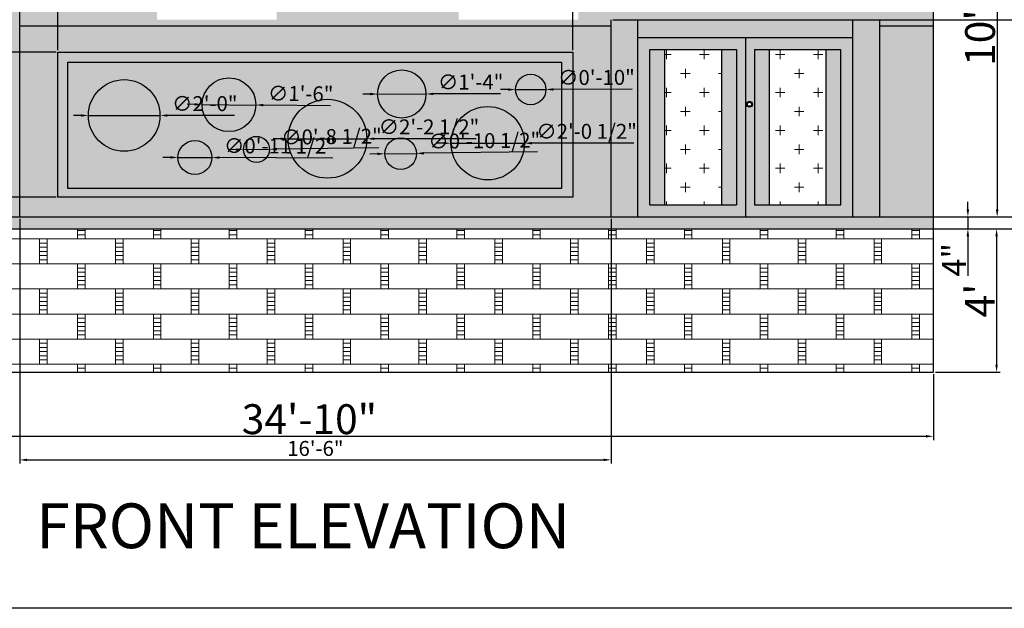
# Model space of a CAD drawing. Units: inches. Extents: x 1662 to 23131, y 1265 to 19127.
# Tile 10 of 26: x 17387 to 17717, y 7742 to 7939. Entities that reach past the tile are written whole.
import ezdxf

# ---------------------------------------------------------------- set-up
doc = ezdxf.new("R2010")
doc.units = ezdxf.units.IN
for name, color, linetype, lineweight in [('A-ANNO-DIMS', 4, 'Continuous', 18), ('A-ANNO-TITL', 7, 'Continuous', 35), ('A-ANNO-TTLB', 7, 'Continuous', 25), ('A-ELEV', 7, 'Continuous', 25), ('A-ELEV-PATT', 8, 'Continuous', 13), ('A-ELEV-SURF-PATT', 252, 'Continuous', 13)]:
    doc.layers.add(name, color=color, linetype=linetype, lineweight=lineweight)
doc.styles.get("Standard").update_dxf_attribs({"font": 'arial.ttf'})
doc.dimstyles.new('ISO-25', dxfattribs={"dimtxt": 5, "dimasz": 2.5, "dimexe": 1.25, "dimexo": 0.625, "dimtad": 1, "dimlunit": 3, "dimtxsty": 'Standard', "dimcen": 2.5, "dimadec": 0, "dimazin": 0, "dimtfac": 1, "dimtmove": 0, "dimatfit": 3, "dimfxl": 1, "dimarcsym": 0})

# ---------------------------------------------------------------- blocks, each defined once
blk = doc.blocks.new('*D78')
at = {"layer": 'A-ANNO-DIMS', "color": 0, "lineweight": -2, "transparency": 16777216}
for p, q in [((17693.88, 7993.16), (17715.8, 7993.16)), ((17714.55, 7990.66), (17714.55, 7875.66)), ((17693.88, 7873.16), (17715.8, 7873.16))]:
    blk.add_line(p, q, dxfattribs=at)
at = {"layer": 'A-ANNO-DIMS', "color": 0, "transparency": 16777216}
for points in [[(17714.13, 7990.66), (17714.97, 7990.66), (17714.55, 7993.16)], [(17714.13, 7875.66), (17714.97, 7875.66), (17714.55, 7873.16)]]:
    blk.add_solid(points, dxfattribs=at)
at = {"layer": 'Defpoints', "color": 0, "transparency": 16777216}
for p in [(17693.26, 7993.16), (17693.26, 7873.16), (17714.55, 7873.16)]:
    blk.add_point(p, dxfattribs=at)
at = {"layer": 'A-ANNO-DIMS', "color": 0, "transparency": 16777216, "insert": (17708.82, 7933.16), "char_height": 5, "attachment_point": 5, "rotation": 90}
blk.add_mtext("{\\H2x;10'}", dxfattribs=at)
blk = doc.blocks.new('*D83')
at = {"layer": 'A-ANNO-DIMS', "color": 0, "lineweight": -2, "transparency": 16777216}
for p, q in [((17693.88, 7869.16), (17715.61, 7869.16)), ((17714.36, 7866.66), (17714.36, 7823.66)), ((17693.88, 7821.16), (17715.61, 7821.16))]:
    blk.add_line(p, q, dxfattribs=at)
at = {"layer": 'A-ANNO-DIMS', "color": 0, "transparency": 16777216}
for points in [[(17713.94, 7866.66), (17714.77, 7866.66), (17714.36, 7869.16)], [(17713.94, 7823.66), (17714.77, 7823.66), (17714.36, 7821.16)]]:
    blk.add_solid(points, dxfattribs=at)
at = {"layer": 'Defpoints', "color": 0, "transparency": 16777216}
for p in [(17693.26, 7869.16), (17693.26, 7821.16), (17714.36, 7821.16)]:
    blk.add_point(p, dxfattribs=at)
at = {"layer": 'A-ANNO-DIMS', "color": 0, "transparency": 16777216, "insert": (17708.73, 7845.16), "char_height": 5, "attachment_point": 5, "rotation": 90}
blk.add_mtext("{\\H2x;4'}", dxfattribs=at)
blk = doc.blocks.new('*D84')
at = {"layer": 'A-ANNO-DIMS', "color": 0, "lineweight": -2, "transparency": 16777216}
for p, q in [((17704.75, 7875.66), (17704.75, 7878.16)), ((17693.88, 7873.16), (17706, 7873.16)), ((17704.75, 7873.16), (17704.75, 7869.16)), ((17693.88, 7869.16), (17706, 7869.16)), ((17704.75, 7866.66), (17704.75, 7853.39))]:
    blk.add_line(p, q, dxfattribs=at)
at = {"layer": 'A-ANNO-DIMS', "color": 0, "transparency": 16777216}
for points in [[(17704.33, 7875.66), (17705.16, 7875.66), (17704.75, 7873.16)], [(17704.33, 7866.66), (17705.16, 7866.66), (17704.75, 7869.16)]]:
    blk.add_solid(points, dxfattribs=at)
at = {"layer": 'Defpoints', "color": 0, "transparency": 16777216}
for p in [(17693.26, 7873.16), (17693.26, 7869.16), (17704.75, 7869.16)]:
    blk.add_point(p, dxfattribs=at)
at = {"layer": 'A-ANNO-DIMS', "color": 0, "transparency": 16777216, "insert": (17700.12, 7858.78), "char_height": 5, "attachment_point": 5, "rotation": 90}
blk.add_mtext('{\\H1.6x;4"}', dxfattribs=at)
blk = doc.blocks.new('*D85')
at = {"layer": 'A-ANNO-DIMS', "color": 0, "lineweight": -2, "transparency": 16777216}
for p, q in [((17275.26, 7820.53), (17275.26, 7798.45)), ((17693.26, 7820.53), (17693.26, 7798.45)), ((17277.76, 7799.7), (17690.76, 7799.7))]:
    blk.add_line(p, q, dxfattribs=at)
at = {"layer": 'A-ANNO-DIMS', "color": 0, "transparency": 16777216}
for points in [[(17277.76, 7800.12), (17277.76, 7799.28), (17275.26, 7799.7)], [(17690.76, 7800.12), (17690.76, 7799.28), (17693.26, 7799.7)]]:
    blk.add_solid(points, dxfattribs=at)
at = {"layer": 'Defpoints', "color": 0, "transparency": 16777216}
for p in [(17275.26, 7821.16), (17693.26, 7821.16), (17693.26, 7799.7)]:
    blk.add_point(p, dxfattribs=at)
at = {"layer": 'A-ANNO-DIMS', "color": 0, "transparency": 16777216, "insert": (17484.26, 7805.43), "char_height": 5, "attachment_point": 5}
blk.add_mtext('{\\H2x;34\'-10"}', dxfattribs=at)
blk = doc.blocks.new('*D237')
at = {"layer": 'A-ANNO-DIMS', "color": 0, "lineweight": -2, "transparency": 16777216}
for p, q in [((17387.26, 7872.53), (17387.26, 7790.56)), ((17585.26, 7872.53), (17585.26, 7790.56)), ((17389.76, 7791.81), (17582.76, 7791.81))]:
    blk.add_line(p, q, dxfattribs=at)
at = {"layer": 'A-ANNO-DIMS', "color": 0, "transparency": 16777216}
for points in [[(17389.76, 7792.23), (17389.76, 7791.39), (17387.26, 7791.81)], [(17582.76, 7792.23), (17582.76, 7791.39), (17585.26, 7791.81)]]:
    blk.add_solid(points, dxfattribs=at)
at = {"layer": 'Defpoints', "color": 0, "transparency": 16777216}
for p in [(17387.26, 7873.16), (17585.26, 7873.16), (17585.26, 7791.81)]:
    blk.add_point(p, dxfattribs=at)
at = {"layer": 'A-ANNO-DIMS', "color": 0, "transparency": 16777216, "insert": (17486.26, 7794.99), "char_height": 5, "attachment_point": 5}
blk.add_mtext('16\'-6"', dxfattribs=at)
blk = doc.blocks.new('*D238')
at = {"layer": 'A-ANNO-DIMS', "color": 0, "lineweight": -2, "transparency": 16777216}
for p, q in [((17585.88, 7939.16), (17789.71, 7939.16)), ((17788.46, 7875.66), (17788.46, 7936.66)), ((17585.88, 7873.16), (17789.71, 7873.16))]:
    blk.add_line(p, q, dxfattribs=at)
at = {"layer": 'A-ANNO-DIMS', "color": 0, "transparency": 16777216}
for points in [[(17788.04, 7936.66), (17788.87, 7936.66), (17788.46, 7939.16)], [(17788.04, 7875.66), (17788.87, 7875.66), (17788.46, 7873.16)]]:
    blk.add_solid(points, dxfattribs=at)
at = {"layer": 'Defpoints', "color": 0, "transparency": 16777216}
for p in [(17585.26, 7939.16), (17788.46, 7939.16), (17585.26, 7873.16)]:
    blk.add_point(p, dxfattribs=at)
at = {"layer": 'A-ANNO-DIMS', "color": 0, "transparency": 16777216, "insert": (17785.28, 7906.16), "char_height": 5, "attachment_point": 5, "rotation": 90}
blk.add_mtext('5\'-6"', dxfattribs=at)
blk = doc.blocks.new('*D239')
at = {"layer": 'A-ANNO-DIMS', "color": 0, "lineweight": -2, "transparency": 16777216}
for p, q in [((17400.05, 7928.94), (17400.05, 8244.76)), ((17402.55, 8243.51), (17569.96, 8243.51)), ((17572.46, 7928.94), (17572.46, 8244.76))]:
    blk.add_line(p, q, dxfattribs=at)
at = {"layer": 'A-ANNO-DIMS', "color": 0, "transparency": 16777216}
for points in [[(17402.55, 8243.93), (17402.55, 8243.09), (17400.05, 8243.51)], [(17569.96, 8243.93), (17569.96, 8243.09), (17572.46, 8243.51)]]:
    blk.add_solid(points, dxfattribs=at)
at = {"layer": 'Defpoints', "color": 0, "transparency": 16777216}
for p in [(17572.46, 8243.51), (17400.05, 7928.32), (17572.46, 7928.32)]:
    blk.add_point(p, dxfattribs=at)
at = {"layer": 'A-ANNO-DIMS', "color": 0, "transparency": 16777216, "insert": (17486.26, 8246.72), "char_height": 5, "attachment_point": 5}
blk.add_mtext('14\'-4 1/2"', dxfattribs=at)
blk = doc.blocks.new('*D240')
at = {"layer": 'A-ANNO-DIMS', "color": 0, "lineweight": -2, "transparency": 16777216}
for p, q in [((17399.43, 7928.32), (17177.82, 7928.32)), ((17179.07, 7882.22), (17179.07, 7925.82)), ((17399.43, 7879.72), (17177.82, 7879.72))]:
    blk.add_line(p, q, dxfattribs=at)
at = {"layer": 'A-ANNO-DIMS', "color": 0, "transparency": 16777216}
for points in [[(17178.65, 7925.82), (17179.48, 7925.82), (17179.07, 7928.32)], [(17178.65, 7882.22), (17179.48, 7882.22), (17179.07, 7879.72)]]:
    blk.add_solid(points, dxfattribs=at)
at = {"layer": 'Defpoints', "color": 0, "transparency": 16777216}
for p in [(17179.07, 7928.32), (17400.05, 7928.32), (17400.05, 7879.72)]:
    blk.add_point(p, dxfattribs=at)
at = {"layer": 'A-ANNO-DIMS', "color": 0, "transparency": 16777216, "insert": (17175.86, 7904.02), "char_height": 5, "attachment_point": 5, "rotation": 90}
blk.add_mtext('4\'-0 1/2"', dxfattribs=at)
blk = doc.blocks.new('*D268')
at = {"layer": 'A-ANNO-DIMS', "color": 0, "lineweight": -2, "transparency": 16777216}
for p, q in [((17407.75, 7907.1), (17405.25, 7907.1)), ((17410.25, 7907.1), (17434.24, 7907.1)), ((17459.22, 7907.1), (17436.74, 7907.1))]:
    blk.add_line(p, q, dxfattribs=at)
at = {"layer": 'A-ANNO-DIMS', "color": 0, "transparency": 16777216}
for points in [[(17407.75, 7907.51), (17407.75, 7906.68), (17410.25, 7907.1)], [(17436.74, 7907.51), (17436.74, 7906.68), (17434.24, 7907.1)]]:
    blk.add_solid(points, dxfattribs=at)
at = {"layer": 'Defpoints', "color": 0, "transparency": 16777216}
for p in [(17410.25, 7907.1), (17434.24, 7907.1)]:
    blk.add_point(p, dxfattribs=at)
at = {"layer": 'A-ANNO-DIMS', "color": 0, "transparency": 16777216, "insert": (17449.23, 7910.42), "char_height": 5, "attachment_point": 5, "rotation": 0}
blk.add_mtext('∅2\'-0"', dxfattribs=at)
blk = doc.blocks.new('*D269')
at = {"layer": 'A-ANNO-DIMS', "color": 0, "lineweight": -2, "transparency": 16777216}
for p, q in [((17437.73, 7893.06), (17435.23, 7893.07)), ((17440.23, 7893.05), (17451.63, 7893)), ((17492.14, 7892.84), (17454.13, 7892.99))]:
    blk.add_line(p, q, dxfattribs=at)
at = {"layer": 'A-ANNO-DIMS', "color": 0, "transparency": 16777216}
for points in [[(17437.74, 7893.47), (17437.73, 7892.64), (17440.23, 7893.05)], [(17454.13, 7893.41), (17454.13, 7892.57), (17451.63, 7893)]]:
    blk.add_solid(points, dxfattribs=at)
at = {"layer": 'Defpoints', "color": 0, "transparency": 16777216}
for p in [(17440.23, 7893.05), (17451.63, 7893)]:
    blk.add_point(p, dxfattribs=at)
at = {"layer": 'A-ANNO-DIMS', "color": 0, "transparency": 16777216, "insert": (17474.4, 7896.23), "char_height": 5, "attachment_point": 5, "rotation": 359.7696}
blk.add_mtext('∅0\'-11 1/2"', dxfattribs=at)
blk = doc.blocks.new('*D270')
at = {"layer": 'A-ANNO-DIMS', "color": 0, "lineweight": -2, "transparency": 16777216}
for p, q in [((17445.83, 7910.81), (17443.33, 7910.83)), ((17448.33, 7910.78), (17466.32, 7910.6)), ((17491.3, 7910.34), (17468.82, 7910.57))]:
    blk.add_line(p, q, dxfattribs=at)
at = {"layer": 'A-ANNO-DIMS', "color": 0, "transparency": 16777216}
for points in [[(17445.83, 7911.23), (17445.83, 7910.39), (17448.33, 7910.78)], [(17468.82, 7910.99), (17468.81, 7910.16), (17466.32, 7910.6)]]:
    blk.add_solid(points, dxfattribs=at)
at = {"layer": 'Defpoints', "color": 0, "transparency": 16777216}
for p in [(17448.33, 7910.78), (17466.32, 7910.6)]:
    blk.add_point(p, dxfattribs=at)
at = {"layer": 'A-ANNO-DIMS', "color": 0, "transparency": 16777216, "insert": (17481.34, 7913.76), "char_height": 5, "attachment_point": 5, "rotation": 359.4142}
blk.add_mtext('∅1\'-6"', dxfattribs=at)
blk = doc.blocks.new('*D271')
at = {"layer": 'A-ANNO-DIMS', "color": 0, "lineweight": -2, "transparency": 16777216}
for p, q in [((17507.53, 7896.26), (17473.4, 7895.83)), ((17459.69, 7895.66), (17457.19, 7895.63)), ((17462.19, 7895.69), (17470.9, 7895.8))]:
    blk.add_line(p, q, dxfattribs=at)
at = {"layer": 'A-ANNO-DIMS', "color": 0, "transparency": 16777216}
for points in [[(17459.69, 7896.07), (17459.7, 7895.24), (17462.19, 7895.69)], [(17473.39, 7896.25), (17473.4, 7895.41), (17470.9, 7895.8)]]:
    blk.add_solid(points, dxfattribs=at)
at = {"layer": 'Defpoints', "color": 0, "transparency": 16777216}
for p in [(17462.19, 7895.69), (17470.9, 7895.8)]:
    blk.add_point(p, dxfattribs=at)
at = {"layer": 'A-ANNO-DIMS', "color": 0, "transparency": 16777216, "insert": (17491.67, 7899.38), "char_height": 5, "attachment_point": 5, "rotation": 0.7249}
blk.add_mtext('∅0\'-8 1/2"', dxfattribs=at)
blk = doc.blocks.new('*D272')
at = {"layer": 'A-ANNO-DIMS', "color": 0, "lineweight": -2, "transparency": 16777216}
for p, q in [((17474.61, 7899.31), (17472.11, 7899.31)), ((17477.11, 7899.31), (17503.5, 7899.31)), ((17540.13, 7899.31), (17506, 7899.31))]:
    blk.add_line(p, q, dxfattribs=at)
at = {"layer": 'A-ANNO-DIMS', "color": 0, "transparency": 16777216}
for points in [[(17474.61, 7899.73), (17474.61, 7898.9), (17477.11, 7899.31)], [(17506, 7899.73), (17506, 7898.89), (17503.5, 7899.31)]]:
    blk.add_solid(points, dxfattribs=at)
at = {"layer": 'Defpoints', "color": 0, "transparency": 16777216}
for p in [(17477.11, 7899.31), (17503.5, 7899.31)]:
    blk.add_point(p, dxfattribs=at)
at = {"layer": 'A-ANNO-DIMS', "color": 0, "transparency": 16777216, "insert": (17524.31, 7902.63), "char_height": 5, "attachment_point": 5, "rotation": 359.9979}
blk.add_mtext('∅2\'-2 1/2"', dxfattribs=at)
blk = doc.blocks.new('*D273')
at = {"layer": 'A-ANNO-DIMS', "color": 0, "lineweight": -2, "transparency": 16777216}
for p, q in [((17504.61, 7914.27), (17502.11, 7914.26)), ((17507.11, 7914.27), (17523.28, 7914.3)), ((17548.26, 7914.34), (17525.78, 7914.3))]:
    blk.add_line(p, q, dxfattribs=at)
at = {"layer": 'A-ANNO-DIMS', "color": 0, "transparency": 16777216}
for points in [[(17504.6, 7914.68), (17504.61, 7913.85), (17507.11, 7914.27)], [(17525.78, 7914.72), (17525.78, 7913.89), (17523.28, 7914.3)]]:
    blk.add_solid(points, dxfattribs=at)
at = {"layer": 'Defpoints', "color": 0, "transparency": 16777216}
for p in [(17507.11, 7914.27), (17523.28, 7914.3)]:
    blk.add_point(p, dxfattribs=at)
at = {"layer": 'A-ANNO-DIMS', "color": 0, "transparency": 16777216, "insert": (17538.26, 7917.64), "char_height": 5, "attachment_point": 5, "rotation": 0.1009}
blk.add_mtext('∅1\'-4"', dxfattribs=at)
blk = doc.blocks.new('*D274')
at = {"layer": 'A-ANNO-DIMS', "color": 0, "lineweight": -2, "transparency": 16777216}
for p, q in [((17507.03, 7894.23), (17504.53, 7894.2)), ((17509.53, 7894.27), (17520.11, 7894.4)), ((17560.63, 7894.92), (17522.61, 7894.43))]:
    blk.add_line(p, q, dxfattribs=at)
at = {"layer": 'A-ANNO-DIMS', "color": 0, "transparency": 16777216}
for points in [[(17507.02, 7894.65), (17507.04, 7893.82), (17509.53, 7894.27)], [(17522.61, 7894.85), (17522.62, 7894.02), (17520.11, 7894.4)]]:
    blk.add_solid(points, dxfattribs=at)
at = {"layer": 'Defpoints', "color": 0, "transparency": 16777216}
for p in [(17509.53, 7894.27), (17520.11, 7894.4)]:
    blk.add_point(p, dxfattribs=at)
at = {"layer": 'A-ANNO-DIMS', "color": 0, "transparency": 16777216, "insert": (17542.83, 7898.01), "char_height": 5, "attachment_point": 5, "rotation": 0.7347}
blk.add_mtext('∅0\'-10 1/2"', dxfattribs=at)
blk = doc.blocks.new('*D275')
at = {"layer": 'A-ANNO-DIMS', "color": 0, "lineweight": -2, "transparency": 16777216}
for p, q in [((17529.18, 7897.81), (17526.68, 7897.81)), ((17531.68, 7897.81), (17556.27, 7897.81)), ((17592.9, 7897.81), (17558.77, 7897.81))]:
    blk.add_line(p, q, dxfattribs=at)
at = {"layer": 'A-ANNO-DIMS', "color": 0, "transparency": 16777216}
for points in [[(17529.18, 7898.23), (17529.18, 7897.4), (17531.68, 7897.81)], [(17558.77, 7898.23), (17558.77, 7897.4), (17556.27, 7897.81)]]:
    blk.add_solid(points, dxfattribs=at)
at = {"layer": 'Defpoints', "color": 0, "transparency": 16777216}
for p in [(17531.68, 7897.81), (17556.27, 7897.81)]:
    blk.add_point(p, dxfattribs=at)
at = {"layer": 'A-ANNO-DIMS', "color": 0, "transparency": 16777216, "insert": (17577.08, 7901.13), "char_height": 5, "attachment_point": 5, "rotation": 359.9996}
blk.add_mtext('∅2\'-0 1/2"', dxfattribs=at)
blk = doc.blocks.new('*D276')
at = {"layer": 'A-ANNO-DIMS', "color": 0, "lineweight": -2, "transparency": 16777216}
for p, q in [((17550.78, 7915.76), (17548.28, 7915.75)), ((17553.28, 7915.77), (17563.46, 7915.8)), ((17592.32, 7915.9), (17565.96, 7915.81))]:
    blk.add_line(p, q, dxfattribs=at)
at = {"layer": 'A-ANNO-DIMS', "color": 0, "transparency": 16777216}
for points in [[(17550.77, 7916.17), (17550.78, 7915.34), (17553.28, 7915.77)], [(17565.96, 7916.23), (17565.96, 7915.39), (17563.46, 7915.8)]]:
    blk.add_solid(points, dxfattribs=at)
at = {"layer": 'Defpoints', "color": 0, "transparency": 16777216}
for p in [(17553.28, 7915.77), (17563.46, 7915.8)]:
    blk.add_point(p, dxfattribs=at)
at = {"layer": 'A-ANNO-DIMS', "color": 0, "transparency": 16777216, "insert": (17580.38, 7919.18), "char_height": 5, "attachment_point": 5, "rotation": 0.1981}
blk.add_mtext('∅0\'-10"', dxfattribs=at)

msp = doc.modelspace()

# ---------------------------------------------------------------- hatches: boundary and pattern name
at = {"layer": 'A-ELEV-PATT'}
h = msp.add_hatch(dxfattribs=at)
h.set_pattern_fill('CROSS', color=256)
h.set_pattern_definition([(0, (0, 78.8975), (6.35, 6.35), [3.175, -9.525]), (90, (1.5875, 77.31), (-6.35, 6.35), [3.175, -9.525])])
h.paths.add_polyline_path([(17603.258, 7877.159), (17622.258, 7877.159), (17622.258, 7929.159), (17603.258, 7929.159)])
h.paths.add_polyline_path([(17638.258, 7877.159), (17657.258, 7877.159), (17657.258, 7929.159), (17638.258, 7929.159)])
h = msp.add_hatch(dxfattribs=at)
h.set_pattern_fill('BRSTONE', color=256)
h.set_pattern_definition([(0, (0, 78.8975), (0, 8.382), []), (90, (22.86, 78.898), (-12.7, 8.382), [8.382, -8.382]), (90, (20.32, 78.898), (-12.7, 8.382), [8.382, -8.382]), (0, (22.86, 80.2945), (12.7, 8.382), [-22.86, 2.54]), (0, (22.86, 81.6915), (12.7, 8.382), [-22.86, 2.54]), (0, (22.86, 83.0885), (12.7, 8.382), [-22.86, 2.54]), (0, (22.86, 84.4855), (12.7, 8.382), [-22.86, 2.54]), (0, (22.86, 85.8825), (12.7, 8.382), [-22.86, 2.54])])
h.paths.add_polyline_path([(17693.258, 7821.159), (17693.258, 7869.159), (17275.258, 7869.159), (17275.258, 7821.159)])
at = {"layer": 'A-ELEV-SURF-PATT'}
h = msp.add_hatch(color=256, dxfattribs=at)
h.dxf.hatch_style = 1
h.paths.add_polyline_path([(17263.258, 8214.159), (17263.258, 8209.159), (17411.258, 8209.159), (17411.258, 8214.159)])
h.paths.add_polyline_path([(17699.258, 8119.159), (17699.258, 8125.159), (17693.258, 8125.159), (17693.258, 8128.159), (17684.258, 8128.159), (17616.758, 8128.159), (17607.758, 8128.159), (17544.758, 8128.159), (17535.758, 8128.159), (17472.758, 8128.159), (17463.758, 8128.159), (17396.258, 8128.159), (17387.258, 8128.159), (17387.258, 8119.159)])
h.paths.add_polyline_path([(17699.258, 7993.159), (17699.258, 7999.159), (17693.258, 7999.159), (17693.258, 8002.159), (17684.258, 8002.159), (17616.758, 8002.159), (17607.758, 8002.159), (17544.758, 8002.159), (17535.758, 8002.159), (17472.758, 8002.159), (17463.758, 8002.159), (17396.258, 8002.159), (17387.258, 8002.159), (17387.258, 7993.159)])
h.paths.add_polyline_path([(17693.258, 7869.159), (17693.258, 7873.159), (17275.258, 7873.159), (17275.258, 7869.159)])
h.paths.add_polyline_path([(17396.258, 8035.159), (17398.258, 8035.159), (17398.258, 8037.159), (17396.258, 8037.159), (17387.258, 8037.159), (17387.258, 8035.159)])
h.paths.add_polyline_path([(17473.258, 8035.159), (17474.758, 8035.159), (17474.758, 8037.159), (17461.758, 8037.159), (17461.758, 8035.159)])
h.paths.add_polyline_path([(17546.758, 8037.159), (17544.758, 8037.159), (17535.758, 8037.159), (17533.758, 8037.159), (17533.758, 8035.159), (17535.758, 8035.159), (17544.758, 8035.159), (17546.758, 8035.159)])
h.paths.add_polyline_path([(17616.758, 8035.159), (17618.758, 8035.159), (17618.758, 8037.159), (17616.758, 8037.159), (17607.758, 8037.159), (17605.758, 8037.159), (17605.758, 8035.159), (17607.758, 8035.159)])
h.paths.add_polyline_path([(17695.258, 8035.159), (17695.258, 8037.159), (17684.258, 8037.159), (17682.258, 8037.159), (17682.258, 8035.159), (17684.258, 8035.159)])
h.paths.add_polyline_path([(17684.258, 8163.159), (17682.258, 8163.159), (17682.258, 8161.159), (17684.258, 8161.159), (17693.258, 8161.159), (17695.258, 8161.159), (17695.258, 8163.159), (17693.258, 8163.159)])
h.paths.add_polyline_path([(17616.758, 8161.159), (17618.758, 8161.159), (17618.758, 8163.159), (17616.758, 8163.159), (17607.758, 8163.159), (17605.758, 8163.159), (17605.758, 8161.159), (17607.758, 8161.159)])
h.paths.add_polyline_path([(17544.758, 8161.159), (17546.758, 8161.159), (17546.758, 8163.159), (17544.758, 8163.159), (17535.758, 8163.159), (17533.758, 8163.159), (17533.758, 8161.159), (17535.758, 8161.159)])
h.paths.add_polyline_path([(17463.758, 8163.159), (17461.758, 8163.159), (17461.758, 8161.159), (17463.758, 8161.159), (17472.758, 8161.159), (17474.758, 8161.159), (17474.758, 8163.159), (17472.758, 8163.159)])
h.paths.add_polyline_path([(17396.258, 8161.159), (17398.258, 8161.159), (17398.258, 8163.159), (17396.258, 8163.159), (17387.258, 8163.159), (17387.258, 8161.159)])
h.paths.add_polyline_path([(17711.258, 8083.159), (17711.258, 8086.159), (17693.258, 8089.159), (17693.258, 8083.159)])
h.paths.add_polyline_path([(17711.258, 7960.159), (17711.258, 7963.159), (17693.258, 7966.159), (17693.258, 7960.159)])
h.paths.add_polyline_path([(17263.258, 7963.159), (17263.258, 7960.159), (17275.258, 7960.159), (17275.258, 7966.159)])
h.paths.add_polyline_path([(17275.258, 8083.159), (17275.258, 8089.159), (17263.258, 8086.159), (17263.258, 8083.159)])
h = msp.add_hatch(color=256, dxfattribs=at)
h.dxf.hatch_style = 1
h.paths.add_polyline_path([(17275.258, 8209.159), (17275.258, 8041.159), (17275.258, 7873.159), (17387.258, 7873.159), (17387.258, 8209.159)])
h.paths.add_polyline_path([(17360.258, 8122.159), (17360.258, 7936.159), (17302.258, 7936.159), (17302.258, 8122.159)], flags=16)
h.paths.add_polyline_path([(17357.258, 8119.159), (17357.258, 7939.159), (17305.258, 7939.159), (17305.258, 8119.159)], flags=0)
h = msp.add_hatch(color=256, dxfattribs=at)
h.dxf.hatch_style = 1
h.paths.add_polyline_path([(17396.258, 8161.159), (17387.258, 8161.159), (17387.258, 8128.159), (17396.258, 8128.159)])
h.paths.add_polyline_path([(17463.758, 8128.159), (17472.758, 8128.159), (17472.758, 8161.159), (17463.758, 8161.159)])
h.paths.add_polyline_path([(17544.758, 8161.159), (17535.758, 8161.159), (17535.758, 8128.159), (17544.758, 8128.159)])
h.paths.add_polyline_path([(17616.758, 8161.159), (17607.758, 8161.159), (17607.758, 8128.159), (17616.758, 8128.159)])
h.paths.add_polyline_path([(17693.258, 8161.159), (17684.258, 8161.159), (17684.258, 8128.159), (17693.258, 8128.159)])
h.paths.add_polyline_path([(17396.258, 8035.159), (17387.258, 8035.159), (17387.258, 8002.159), (17396.258, 8002.159)])
h.paths.add_polyline_path([(17472.758, 8035.159), (17463.758, 8035.159), (17463.758, 8002.159), (17472.758, 8002.159)])
h.paths.add_polyline_path([(17544.758, 8035.159), (17535.758, 8035.159), (17535.758, 8002.159), (17544.758, 8002.159)])
h.paths.add_polyline_path([(17616.758, 8035.159), (17607.758, 8035.159), (17607.758, 8002.159), (17616.758, 8002.159)])
h.paths.add_polyline_path([(17684.258, 8002.159), (17693.258, 8002.159), (17693.258, 8035.159), (17684.258, 8035.159)])
h.paths.add_polyline_path([(17666.258, 7873.159), (17675.258, 7873.159), (17675.258, 7939.159), (17666.258, 7939.159)])
h.paths.add_polyline_path([(17594.258, 7939.159), (17585.258, 7939.159), (17585.258, 7873.159), (17594.258, 7873.159)])
h = msp.add_hatch(color=256, dxfattribs=at)
h.dxf.hatch_style = 1
h.paths.add_polyline_path([(17618.758, 8037.159), (17618.758, 8035.159), (17616.758, 8035.159), (17616.758, 8033.159), (17684.258, 8033.159), (17684.258, 8035.159), (17682.258, 8035.159), (17682.258, 8037.159), (17684.258, 8037.159), (17693.258, 8037.159), (17693.258, 8119.159), (17387.258, 8119.159), (17387.258, 8037.159), (17396.258, 8037.159), (17398.258, 8037.159), (17398.258, 8035.159), (17396.258, 8035.159), (17396.258, 8033.159), (17463.758, 8033.159), (17463.758, 8035.159), (17433.258, 8035.159), (17433.258, 8083.159), (17421.258, 8083.159), (17421.258, 8086.159), (17433.258, 8092.159), (17473.258, 8092.159), (17485.258, 8086.159), (17485.258, 8083.159), (17473.258, 8083.159), (17473.258, 8037.159), (17474.758, 8037.159), (17474.758, 8035.159), (17472.758, 8035.159), (17472.758, 8033.159), (17534.258, 8033.159), (17534.258, 8035.159), (17533.758, 8035.159), (17533.758, 8037.159), (17534.258, 8083.159), (17574.258, 8083.159), (17574.258, 8033.159), (17607.758, 8033.159), (17607.758, 8035.159), (17605.758, 8035.159), (17605.758, 8037.159), (17607.758, 8037.159), (17616.758, 8037.159)])
h.paths.add_polyline_path([(17387.258, 7993.159), (17387.258, 7939.159), (17433.258, 7939.159), (17433.258, 7960.159), (17421.258, 7960.159), (17421.258, 7963.159), (17433.258, 7969.159), (17473.258, 7969.159), (17485.258, 7963.159), (17485.258, 7960.159), (17473.258, 7960.159), (17473.258, 7939.159), (17534.258, 7939.159), (17534.258, 7960.159), (17574.258, 7960.159), (17574.258, 7939.159), (17583.258, 7939.159), (17583.258, 7941.159), (17596.258, 7941.159), (17596.258, 7939.159), (17594.258, 7939.159), (17594.258, 7933.159), (17666.258, 7933.159), (17666.258, 7939.159), (17664.258, 7939.159), (17664.258, 7941.159), (17677.258, 7941.159), (17677.258, 7939.159), (17693.258, 7939.159), (17693.258, 7993.159)])
h.paths.add_polyline_path([(17675.258, 7873.159), (17693.258, 7873.159), (17693.258, 7937.159), (17675.258, 7937.159)])
h.paths.add_polyline_path([(17387.258, 7873.159), (17585.258, 7873.159), (17585.258, 7937.159), (17387.258, 7937.159)])
h.paths.add_polyline_path([(17400.054, 7928.315), (17572.458, 7928.315), (17572.458, 7879.721), (17400.054, 7879.721)], flags=16)
h.paths.add_polyline_path([(17403.392, 7924.944), (17568.667, 7924.944), (17568.667, 7882.701), (17403.392, 7882.701)], flags=0)
h.paths.add_polyline_path([(17434.237, 7907.098, -1), (17410.251, 7907.098, -1)], flags=0)
h.paths.add_polyline_path([(17451.627, 7893.022, -1), (17440.234, 7893.022, -1)], flags=0)
h.paths.add_polyline_path([(17466.319, 7910.692, -1), (17448.329, 7910.692, -1)], flags=0)
h.paths.add_polyline_path([(17470.897, 7895.745, -1), (17462.194, 7895.745, -1)], flags=0)
h.paths.add_polyline_path([(17503.498, 7899.311, -1), (17477.113, 7899.311, -1)], flags=0)
h.paths.add_polyline_path([(17523.277, 7914.286, -1), (17507.105, 7914.286, -1)], flags=0)
h.paths.add_polyline_path([(17520.114, 7894.334, -1), (17509.529, 7894.334, -1)], flags=0)
h.paths.add_polyline_path([(17556.268, 7897.814, -1), (17531.682, 7897.814, -1)], flags=0)
h.paths.add_polyline_path([(17563.458, 7915.783, -1), (17553.276, 7915.783, -1)], flags=0)
h = msp.add_hatch(color=256, dxfattribs=at)
h.dxf.hatch_style = 1
h.paths.add_polyline_path([(17596.258, 7941.159), (17583.258, 7941.159), (17583.258, 7939.159), (17596.258, 7939.159)])
h.paths.add_polyline_path([(17585.258, 7939.159), (17583.258, 7939.159), (17387.258, 7939.159), (17387.258, 7937.159), (17585.258, 7937.159)])
h.paths.add_polyline_path([(17693.258, 7939.159), (17675.258, 7939.159), (17675.258, 7937.159), (17693.258, 7937.159)])
h.paths.add_polyline_path([(17677.258, 7941.159), (17664.258, 7941.159), (17664.258, 7939.159), (17677.258, 7939.159)])
h = msp.add_hatch(color=256, dxfattribs=at)
h.dxf.hatch_style = 1
h.paths.add_polyline_path([(17594.258, 7933.159), (17594.258, 7873.159), (17630.258, 7873.159), (17630.258, 7933.159)])
h.paths.add_polyline_path([(17627.258, 7929.159), (17627.258, 7877.159), (17598.258, 7877.159), (17598.258, 7929.159)], flags=16)
h.paths.add_polyline_path([(17630.258, 7933.159), (17630.258, 7873.159), (17666.258, 7873.159), (17666.258, 7933.159)])
h.paths.add_polyline_path([(17662.258, 7929.159), (17662.258, 7877.159), (17633.258, 7877.159), (17633.258, 7929.159)], flags=16)
h.paths.add_polyline_path([(17632.605, 7910.842, -1), (17630.664, 7910.842, -1)], flags=16)
h.paths.add_polyline_path([(17632.317, 7910.842, -1), (17630.952, 7910.842, -1)], flags=0)
h = msp.add_hatch(color=256, dxfattribs=at)
h.dxf.hatch_style = 1
h.paths.add_polyline_path([(17622.258, 7877.159), (17627.258, 7877.159), (17627.258, 7929.159), (17622.258, 7929.159)])
h.paths.add_polyline_path([(17603.258, 7929.159), (17598.258, 7929.159), (17598.258, 7877.159), (17603.258, 7877.159)])
h.paths.add_polyline_path([(17638.258, 7929.159), (17633.258, 7929.159), (17633.258, 7877.159), (17638.258, 7877.159)])
h.paths.add_polyline_path([(17662.258, 7929.159), (17657.258, 7929.159), (17657.258, 7877.159), (17662.258, 7877.159)])
h = msp.add_hatch(color=256, dxfattribs=at)
h.dxf.hatch_style = 1
h.paths.add_polyline_path([(17400.054, 7879.721), (17572.458, 7879.721), (17572.458, 7928.315), (17400.054, 7928.315)])
h.paths.add_polyline_path([(17403.392, 7924.944), (17568.667, 7924.944), (17568.667, 7882.701), (17403.392, 7882.701)], flags=16)
h.paths.add_polyline_path([(17410.251, 7907.098, -1), (17434.237, 7907.098, -1)], flags=0)
h.paths.add_polyline_path([(17440.234, 7893.022, -1), (17451.627, 7893.022, -1)], flags=0)
h.paths.add_polyline_path([(17448.329, 7910.692, -1), (17466.319, 7910.692, -1)], flags=0)
h.paths.add_polyline_path([(17462.194, 7895.745, -1), (17470.897, 7895.745, -1)], flags=0)
h.paths.add_polyline_path([(17477.113, 7899.311, -1), (17503.498, 7899.311, -1)], flags=0)
h.paths.add_polyline_path([(17520.114, 7894.334, -1), (17509.529, 7894.334, -1)], flags=0)
h.paths.add_polyline_path([(17507.105, 7914.286, -1), (17523.277, 7914.286, -1)], flags=0)
h.paths.add_polyline_path([(17531.682, 7897.814, -1), (17556.268, 7897.814, -1)], flags=0)
h.paths.add_polyline_path([(17553.276, 7915.783, -1), (17563.458, 7915.783, -1)], flags=0)
h = msp.add_hatch(color=256, dxfattribs=at)
h.dxf.hatch_style = 1
h.paths.add_polyline_path([(17568.667, 7882.701), (17568.667, 7924.944), (17403.392, 7924.944), (17403.392, 7882.701)])
h.paths.add_polyline_path([(17410.251, 7907.098, -1), (17434.237, 7907.098, -1)], flags=16)
h.paths.add_polyline_path([(17440.234, 7893.022, -1), (17451.627, 7893.022, -1)], flags=16)
h.paths.add_polyline_path([(17448.329, 7910.692, -1), (17466.319, 7910.692, -1)], flags=16)
h.paths.add_polyline_path([(17462.194, 7895.745, -1), (17470.897, 7895.745, -1)], flags=16)
h.paths.add_polyline_path([(17477.113, 7899.311, -1), (17503.498, 7899.311, -1)], flags=16)
h.paths.add_polyline_path([(17520.114, 7894.334, -1), (17509.529, 7894.334, -1)], flags=16)
h.paths.add_polyline_path([(17507.105, 7914.286, -1), (17523.277, 7914.286, -1)], flags=16)
h.paths.add_polyline_path([(17531.682, 7897.814, -1), (17556.268, 7897.814, -1)], flags=16)
h.paths.add_polyline_path([(17553.276, 7915.783, -1), (17563.458, 7915.783, -1)], flags=16)
h = msp.add_hatch(color=256, dxfattribs=at)
h.dxf.hatch_style = 1
h.paths.add_polyline_path([(17410.251, 7907.098, 1), (17434.237, 7907.098, 1)])
h.paths.add_polyline_path([(17448.329, 7910.692, 1), (17466.319, 7910.692, 1)])
h.paths.add_polyline_path([(17440.234, 7893.022, 1), (17451.627, 7893.022, 1)])
h.paths.add_polyline_path([(17462.194, 7895.745, 1), (17470.897, 7895.745, 1)])
h.paths.add_polyline_path([(17503.498, 7899.311, 1), (17477.113, 7899.311, 1)])
h.paths.add_polyline_path([(17507.105, 7914.286, 1), (17523.277, 7914.286, 1)])
h.paths.add_polyline_path([(17520.114, 7894.334, 1), (17509.529, 7894.334, 1)])
h.paths.add_polyline_path([(17556.268, 7897.814, 1), (17531.682, 7897.814, 1)])
h.paths.add_polyline_path([(17563.458, 7915.783, 1), (17553.276, 7915.783, 1)])
h = msp.add_hatch(color=256, dxfattribs=at)
h.dxf.hatch_style = 1
h.paths.add_polyline_path([(17632.605, 7910.842, 1), (17630.664, 7910.842, 1)])
h.paths.add_polyline_path([(17632.317, 7910.842, 1), (17630.952, 7910.842, 1)], flags=16)

# ---------------------------------------------------------------- linework, layer by layer
at = {"layer": 'A-ANNO-TTLB'}
msp.add_lwpolyline([(17164.976, 8731.935), (18265.142, 8731.935), (18265.142, 7742.121), (17164.976, 7742.121)], close=True, dxfattribs=at)
at = {"layer": 'A-ELEV'}
for p, q in [((17387.258, 7873.159), (17387.258, 8209.159)), ((17693.258, 7821.159), (17693.258, 7993.159)), ((17585.258, 7873.159), (17585.258, 7939.159)), ((17594.258, 7873.159), (17594.258, 7939.159)), ((17666.258, 7873.159), (17666.258, 7939.159)), ((17675.258, 7873.159), (17675.258, 7939.159)), ((17387.258, 7937.159), (17585.258, 7937.159)), ((17675.258, 7937.159), (17693.258, 7937.159)), ((17594.258, 7933.159), (17666.258, 7933.159)), ((17630.258, 7933.159), (17630.258, 7873.159)), ((17598.258, 7929.159), (17627.258, 7929.159)), ((17598.258, 7877.159), (17598.258, 7929.159)), ((17603.258, 7877.159), (17603.258, 7929.159)), ((17622.258, 7929.159), (17622.258, 7877.159)), ((17627.258, 7929.159), (17627.258, 7877.159)), ((17633.258, 7929.159), (17633.258, 7877.159)), ((17633.258, 7929.159), (17662.258, 7929.159)), ((17638.258, 7929.159), (17638.258, 7877.159)), ((17657.258, 7877.159), (17657.258, 7929.159)), ((17662.258, 7877.159), (17662.258, 7929.159)), ((17598.258, 7877.159), (17627.258, 7877.159)), ((17633.258, 7877.159), (17662.258, 7877.159)), ((17275.258, 7873.159), (17693.258, 7873.159)), ((17275.258, 7869.159), (17693.258, 7869.159)), ((17693.258, 7869.159), (17759.108, 7869.159)), ((17275.258, 7821.159), (17693.258, 7821.159))]:
    msp.add_line(p, q, dxfattribs=at)
for points in [[(17400.054, 7928.315), (17572.458, 7928.315), (17572.458, 7879.721), (17400.054, 7879.721)], [(17403.392, 7924.944), (17568.667, 7924.944), (17568.667, 7882.701), (17403.392, 7882.701)]]:
    msp.add_lwpolyline(points, close=True, dxfattribs=at)
for centre, radius in [((17515.191, 7914.286), 8.086), ((17422.244, 7907.098), 11.993), ((17457.324, 7910.692), 8.995), ((17558.367, 7915.783), 5.091), ((17490.305, 7899.311), 13.193), ((17543.975, 7897.814), 12.293), ((17631.634, 7910.842), 0.971), ((17631.634, 7910.842), 0.682), ((17466.545, 7895.745), 4.352), ((17514.822, 7894.334), 5.292), ((17445.931, 7893.022), 5.697)]:
    msp.add_circle(centre, radius, dxfattribs=at)

# ---------------------------------------------------------------- texts
at = {"layer": 'A-ANNO-TITL', "insert": (17392.778, 7777.239), "char_height": 15, "attachment_point": 1}
msp.add_mtext_dynamic_manual_height_columns('FRONT ELEVATION', width=1142.59551, gutter_width=12.5, heights=[0], dxfattribs=at)

# ---------------------------------------------------------------- dimensions: what is measured, and where the dimension line sits
at = {"layer": 'A-ANNO-DIMS'}
for base, p1, p2, picture, middle in [((17572.458, 8243.509), (17400.054, 7928.315), (17572.458, 7928.315), '*D239', (17486.256, 8246.72)), ((17585.258, 7791.809), (17387.258, 7873.159), (17585.258, 7873.159), '*D237', (17486.258, 7794.987))]:
    dim = msp.add_linear_dim(base=base, p1=p1, p2=p2, dimstyle='ISO-25', override={"dimdec": 1, "dimlfac": 1, "dimrnd": 0, "dimzin": 1, "dimdsep": 46, "dimlunit": 4, "dimfrac": 2}, dxfattribs=at)
    dim.commit()
    dim.dimension.update_dxf_attribs({"geometry": picture, "text_midpoint": middle})
for base, p1, p2, text, picture, middle in [((17714.55, 7873.159), (17693.258, 7993.159), (17693.258, 7873.159), '{\\H2x;<>}', '*D78', (17708.819, 7933.159)), ((17704.746, 7869.159), (17693.258, 7873.159), (17693.258, 7869.159), '{\\H1.6x;4"}', '*D84', (17700.121, 7858.776)), ((17714.358, 7821.159), (17693.258, 7869.159), (17693.258, 7821.159), '{\\H2x;<>}', '*D83', (17708.733, 7845.159))]:
    dim = msp.add_linear_dim(base=base, p1=p1, p2=p2, angle=90, text=text, dimstyle='ISO-25', override={"dimclrd": 0, "dimclre": 0, "dimclrt": 0}, dxfattribs=at)
    dim.commit()
    dim.dimension.update_dxf_attribs({"geometry": picture, "text_midpoint": middle})
for base, p1, p2, picture, middle in [((17788.458, 7939.159), (17585.258, 7873.159), (17585.258, 7939.159), '*D238', (17785.28, 7906.159)), ((17179.066, 7928.315), (17400.054, 7879.721), (17400.054, 7928.315), '*D240', (17175.856, 7904.018))]:
    dim = msp.add_linear_dim(base=base, p1=p1, p2=p2, angle=90, dimstyle='ISO-25', override={"dimdec": 1, "dimlfac": 1, "dimrnd": 0, "dimzin": 1, "dimdsep": 46, "dimlunit": 4, "dimfrac": 2}, dxfattribs=at)
    dim.commit()
    dim.dimension.update_dxf_attribs({"geometry": picture, "text_midpoint": middle})
for p1, p2, picture, middle in [((17553.276, 7915.765), (17563.458, 7915.801), '*D276', (17580.391, 7915.859)), ((17507.105, 7914.271), (17523.277, 7914.3), '*D273', (17538.268, 7914.326)), ((17448.33, 7910.784), (17466.319, 7910.6), '*D270', (17481.308, 7910.447)), ((17410.251, 7907.098), (17434.237, 7907.098), '*D268', (17449.228, 7907.098)), ((17477.113, 7899.312), (17503.498, 7899.311), '*D272', (17524.314, 7899.31)), ((17531.682, 7897.814), (17556.268, 7897.814), '*D275', (17577.084, 7897.814)), ((17440.234, 7893.045), (17451.627, 7892.999), '*D269', (17474.385, 7892.908))]:
    dim = msp.add_diameter_dim_2p(p1=p1, p2=p2, dimstyle='ISO-25', override={"dimdec": 1, "dimlfac": 1, "dimrnd": 0, "dimzin": 1, "dimdsep": 46, "dimlunit": 4, "dimfrac": 2}, dxfattribs=at)
    dim.commit()
    dim.dimension.update_dxf_attribs({"geometry": picture, "text_midpoint": middle})
for p1, p2, picture, middle in [((17462.194, 7895.69), (17470.897, 7895.8), '*D271', (17491.711, 7896.063)), ((17509.53, 7894.266), (17520.114, 7894.401), '*D274', (17542.87, 7894.693))]:
    dim = msp.add_diameter_dim_2p(p1=p1, p2=p2, dimstyle='ISO-25', override={"dimdec": 1, "dimlfac": 1, "dimrnd": 0, "dimzin": 1, "dimdsep": 46, "dimlunit": 4, "dimfrac": 2}, dxfattribs=at)
    dim.commit()
    dim.dimension.update_dxf_attribs({"geometry": picture, "text_midpoint": middle, "dimtype": 163})
dim = msp.add_linear_dim(base=(17693.258, 7799.701), p1=(17275.258, 7821.159), p2=(17693.258, 7821.159), text='{\\H2x;<>}', dimstyle='ISO-25', override={"dimclrd": 0, "dimclre": 0, "dimclrt": 0}, dxfattribs=at)
dim.commit()
dim.dimension.update_dxf_attribs({"geometry": '*D85', "text_midpoint": (17484.258, 7805.435)})

doc.saveas('drawing.dxf')
